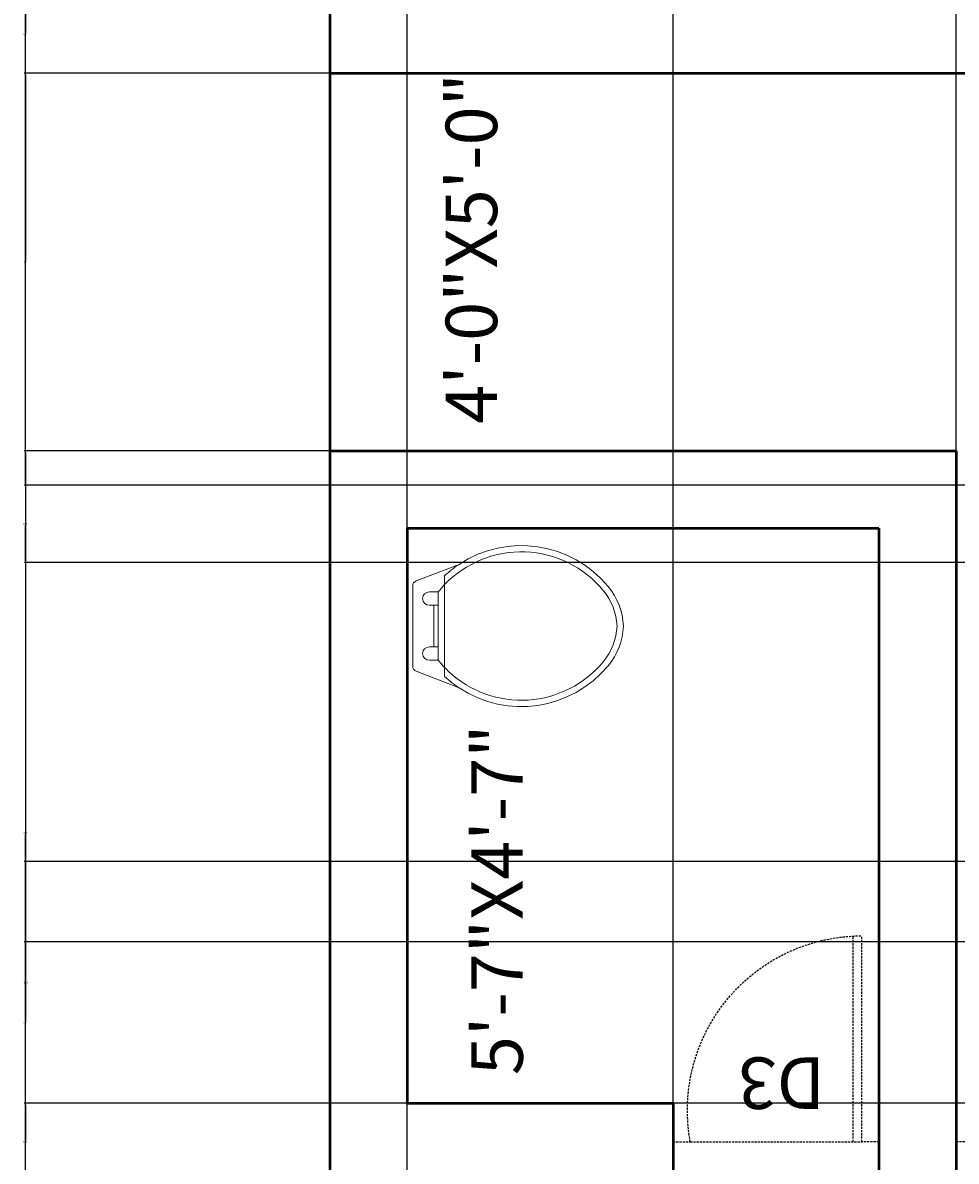
# Model space of a CAD drawing. Units: inches. Extents: x 3 to 576, y -689 to 51.
# Tile 14 of 21: x 3 to 111, y -261 to -128. Entities that reach past the tile are written whole.
import ezdxf

# ---------------------------------------------------------------- set-up
doc = ezdxf.new("R2010")
doc.units = ezdxf.units.IN
doc.header["$MEASUREMENT"] = 0
doc.linetypes.add('DASHED2', pattern=[0.375, 0.25, -0.125])
for name, color, linetype, lineweight in [('A-ANNO-DIMS', 2, 'Continuous', 18), ('A-ANNO-TEXT', 3, 'Continuous', 18), ('A-AREA-IDEN', 7, 'Continuous', 18), ('A-DOOR', 4, 'DASHED2', 25), ('A-FLOR-FIXT', 9, 'Continuous', 18), ('A-WALL', 7, 'Continuous', 50)]:
    doc.layers.add(name, color=color, linetype=linetype, lineweight=lineweight)
doc.styles.get("Standard").update_dxf_attribs({"font": 'arial.ttf'})
doc.dimstyles.get("Standard").update_dxf_attribs({"dimtxt": 0.18, "dimasz": 0.18, "dimexe": 0.18, "dimexo": 0.0625, "dimgap": 0.09, "dimtad": 0, "dimtih": 1, "dimtoh": 1, "dimdec": 0, "dimzin": 0, "dimdsep": 46, "dimlunit": 3, "dimtxsty": 'Standard', "dimcen": 0.09, "dimadec": 0, "dimazin": 0, "dimtfac": 1, "dimtdec": 0, "dimtofl": 0, "dimtmove": 0, "dimatfit": 3, "dimfxl": 1, "dimtolj": 1, "dimtzin": 0, "dimarcsym": 0})

# ---------------------------------------------------------------- blocks, each defined once
blk = doc.blocks.new('WC')
for p, q in [((3.72, 14.21), (3.72, 15.24)), ((3.72, 14.21), (3.72, 9.38)), ((3.72, 4.55), (3.72, 9.38)), ((3.72, 3.52), (3.72, 4.55))]:
    blk.add_line(p, q)
for points in [[(5.4, 16.57, -0.383919), (22.78, 13.99, -0.163732), (24.55, 9.38, -0.359733)], [(3.72, 14.21, -0.448546), (22.21, 13.53, -0.162618), (23.81, 9.38, -0.470877)], [(0, 9.38), (0, 14.07, -0.31031), (0.39, 14.64), (5.4, 16.57, -0.209071)], [(3.72, 15.24, -0.040937), (5.4, 16.57, -0.163732)], [(2.98, 13.36), (1.94, 13.36, 1), (1.94, 11.8), (2.48, 11.8)], [(2.98, 13.36, -0.022712), (3.72, 14.21, -0.162618)], [(2.98, 9.38), (2.98, 13.36, -0.476108)], [(0, 9.38), (0, 4.69, 0.31031), (0.39, 4.12), (5.4, 2.19, 0.209071)], [(2.98, 9.38), (2.98, 5.4, 0.022712)], [(4.22, 4.06, 0.431639), (22.21, 5.23, 0.162618), (23.81, 9.38, 0.470877)], [(5.4, 2.19, 0.383919), (22.78, 4.76, 0.163732), (24.55, 9.38, 0.359733)], [(2.98, 5.4), (1.94, 5.4, -1), (1.94, 6.96), (2.48, 6.96)], [(2.98, 5.4, 0.022712), (3.72, 4.55, 0.162618)], [(3.72, 4.55, 0.014165), (4.22, 4.06, 0.162618)], [(3.72, 3.52, 0.040937), (5.4, 2.19, 0.163732)]]:
    blk.add_lwpolyline(points, format="xyb")
for points in [[(2.48, 11.8), (2.48, 6.96)], [(2.48, 11.8), (2.98, 11.8)], [(2.48, 6.96), (2.98, 6.96)]]:
    blk.add_lwpolyline(points)
blk = doc.blocks.new('DOOR-SWING-750')
for p, q in [((24, 24), (24, 22)), ((24, 22), (24, 2)), ((24, 2), (0, 2)), ((24, 0), (24, 2))]:
    blk.add_line(p, q)
blk.add_arc((20.33, 2), 20.33, 79.6111, 180)
blk = doc.blocks.new('DOOR-900')
for p, q in [((34, 36), (0, 36)), ((2, 36), (2, 0)), ((36, 36), (34, 36))]:
    blk.add_line(p, q)
blk.add_arc((2, 32.22), 32.22, 270, 6.7329)
blk = doc.blocks.new('*D55')
at = {"layer": 'A-ANNO-DIMS', "color": 0, "lineweight": -2, "transparency": 16777216}
for p, q in [((47.23, -125.31), (2.66, -125.31)), ((2.84, -125.49), (2.84, -129.63)), ((2.84, -134.13), (2.84, -129.99)), ((38.23, -134.31), (2.66, -134.31))]:
    blk.add_line(p, q, dxfattribs=at)
at = {"layer": 'A-ANNO-DIMS', "color": 0, "transparency": 16777216}
for points in [[(2.81, -125.49), (2.87, -125.49), (2.84, -125.31)], [(2.81, -134.13), (2.87, -134.13), (2.84, -134.31)]]:
    blk.add_solid(points, dxfattribs=at)
at = {"layer": 'Defpoints', "color": 0, "transparency": 16777216}
for p in [(47.29, -125.31), (2.84, -134.31), (38.29, -134.31)]:
    blk.add_point(p, dxfattribs=at)
at = {"layer": 'A-ANNO-DIMS', "color": 0, "transparency": 16777216, "insert": (2.84, -129.81), "char_height": 0.18, "attachment_point": 5}
blk.add_mtext('\\A1;0\'-9"', dxfattribs=at)
blk = doc.blocks.new('*D56')
at = {"layer": 'A-ANNO-DIMS', "color": 0, "lineweight": -2, "transparency": 16777216}
for p, q in [((38.23, -134.31), (2.66, -134.31)), ((2.84, -134.49), (2.84, -156.13)), ((2.84, -178.13), (2.84, -156.49)), ((38.23, -178.31), (2.66, -178.31))]:
    blk.add_line(p, q, dxfattribs=at)
at = {"layer": 'A-ANNO-DIMS', "color": 0, "transparency": 16777216}
for points in [[(2.81, -134.49), (2.87, -134.49), (2.84, -134.31)], [(2.81, -178.13), (2.87, -178.13), (2.84, -178.31)]]:
    blk.add_solid(points, dxfattribs=at)
at = {"layer": 'Defpoints', "color": 0, "transparency": 16777216}
for p in [(38.29, -134.31), (2.84, -178.31), (38.29, -178.31)]:
    blk.add_point(p, dxfattribs=at)
at = {"layer": 'A-ANNO-DIMS', "color": 0, "transparency": 16777216, "insert": (2.84, -156.31), "char_height": 0.18, "attachment_point": 5}
blk.add_mtext('\\A1;3\'-8"', dxfattribs=at)
blk = doc.blocks.new('*D57')
at = {"layer": 'A-ANNO-DIMS', "color": 0, "lineweight": -2, "transparency": 16777216}
for p, q in [((38.23, -178.31), (2.66, -178.31)), ((2.84, -178.49), (2.84, -240.13)), ((2.84, -302.13), (2.84, -240.49)), ((47.23, -302.31), (2.66, -302.31))]:
    blk.add_line(p, q, dxfattribs=at)
at = {"layer": 'A-ANNO-DIMS', "color": 0, "transparency": 16777216}
for points in [[(2.81, -178.49), (2.87, -178.49), (2.84, -178.31)], [(2.81, -302.13), (2.87, -302.13), (2.84, -302.31)]]:
    blk.add_solid(points, dxfattribs=at)
at = {"layer": 'Defpoints', "color": 0, "transparency": 16777216}
for p in [(38.29, -178.31), (2.84, -302.31), (47.29, -302.31)]:
    blk.add_point(p, dxfattribs=at)
at = {"layer": 'A-ANNO-DIMS', "color": 0, "transparency": 16777216, "insert": (2.84, -240.31), "char_height": 0.18, "attachment_point": 5}
blk.add_mtext('\\A1;10\'-4"', dxfattribs=at)
blk = doc.blocks.new('*D65')
at = {"layer": 'A-ANNO-DIMS', "color": 0, "lineweight": -2, "transparency": 16777216}
for p, q in [((531.23, -50.31), (2.66, -50.31)), ((2.84, -50.49), (2.84, -116.13)), ((2.84, -182.13), (2.84, -116.49)), ((531.23, -182.31), (2.66, -182.31))]:
    blk.add_line(p, q, dxfattribs=at)
at = {"layer": 'A-ANNO-DIMS', "color": 0, "transparency": 16777216}
for points in [[(2.81, -50.49), (2.87, -50.49), (2.84, -50.31)], [(2.81, -182.13), (2.87, -182.13), (2.84, -182.31)]]:
    blk.add_solid(points, dxfattribs=at)
at = {"layer": 'Defpoints', "color": 0, "transparency": 16777216}
for p in [(531.29, -50.31), (2.84, -182.31), (531.29, -182.31)]:
    blk.add_point(p, dxfattribs=at)
at = {"layer": 'A-ANNO-DIMS', "color": 0, "transparency": 16777216, "insert": (2.84, -116.31), "char_height": 0.18, "attachment_point": 5}
blk.add_mtext('\\A1;11\'-0"', dxfattribs=at)
blk = doc.blocks.new('*D66')
at = {"layer": 'A-ANNO-DIMS', "color": 0, "lineweight": -2, "transparency": 16777216}
for p, q in [((531.23, -182.31), (2.66, -182.31)), ((2.84, -182.49), (2.84, -186.63)), ((2.84, -191.13), (2.84, -186.99)), ((531.23, -191.31), (2.66, -191.31))]:
    blk.add_line(p, q, dxfattribs=at)
at = {"layer": 'A-ANNO-DIMS', "color": 0, "transparency": 16777216}
for points in [[(2.81, -182.49), (2.87, -182.49), (2.84, -182.31)], [(2.81, -191.13), (2.87, -191.13), (2.84, -191.31)]]:
    blk.add_solid(points, dxfattribs=at)
at = {"layer": 'Defpoints', "color": 0, "transparency": 16777216}
for p in [(531.29, -182.31), (2.84, -191.31), (531.29, -191.31)]:
    blk.add_point(p, dxfattribs=at)
at = {"layer": 'A-ANNO-DIMS', "color": 0, "transparency": 16777216, "insert": (2.84, -186.81), "char_height": 0.18, "attachment_point": 5}
blk.add_mtext('\\A1;0\'-9"', dxfattribs=at)
blk = doc.blocks.new('*D67')
at = {"layer": 'A-ANNO-DIMS', "color": 0, "lineweight": -2, "transparency": 16777216}
for p, q in [((531.23, -191.31), (2.66, -191.31)), ((2.84, -191.49), (2.84, -222.63)), ((2.84, -254.13), (2.84, -222.99)), ((531.23, -254.31), (2.66, -254.31))]:
    blk.add_line(p, q, dxfattribs=at)
at = {"layer": 'A-ANNO-DIMS', "color": 0, "transparency": 16777216}
for points in [[(2.81, -191.49), (2.87, -191.49), (2.84, -191.31)], [(2.81, -254.13), (2.87, -254.13), (2.84, -254.31)]]:
    blk.add_solid(points, dxfattribs=at)
at = {"layer": 'Defpoints', "color": 0, "transparency": 16777216}
for p in [(531.29, -191.31), (2.84, -254.31), (531.29, -254.31)]:
    blk.add_point(p, dxfattribs=at)
at = {"layer": 'A-ANNO-DIMS', "color": 0, "transparency": 16777216, "insert": (2.84, -222.81), "char_height": 0.18, "attachment_point": 5}
blk.add_mtext('\\A1;5\'-3"', dxfattribs=at)
blk = doc.blocks.new('*D68')
at = {"layer": 'A-ANNO-DIMS', "color": 0, "lineweight": -2, "transparency": 16777216}
for p, q in [((531.23, -254.31), (2.66, -254.31)), ((2.84, -254.49), (2.84, -258.63)), ((2.84, -263.13), (2.84, -258.99)), ((531.23, -263.31), (2.66, -263.31))]:
    blk.add_line(p, q, dxfattribs=at)
at = {"layer": 'A-ANNO-DIMS', "color": 0, "transparency": 16777216}
for points in [[(2.81, -254.49), (2.87, -254.49), (2.84, -254.31)], [(2.81, -263.13), (2.87, -263.13), (2.84, -263.31)]]:
    blk.add_solid(points, dxfattribs=at)
at = {"layer": 'Defpoints', "color": 0, "transparency": 16777216}
for p in [(531.29, -254.31), (2.84, -263.31), (531.29, -263.31)]:
    blk.add_point(p, dxfattribs=at)
at = {"layer": 'A-ANNO-DIMS', "color": 0, "transparency": 16777216, "insert": (2.84, -258.81), "char_height": 0.18, "attachment_point": 5}
blk.add_mtext('\\A1;0\'-9"', dxfattribs=at)
blk = doc.blocks.new('*D89')
at = {"layer": 'A-ANNO-DIMS', "color": 0, "lineweight": -2, "transparency": 16777216}
for p, q in [((170.74, -226.15), (2.66, -226.15)), ((2.84, -226.33), (2.84, -240.05)), ((2.84, -254.13), (2.84, -240.41)), ((170.74, -254.31), (2.66, -254.31))]:
    blk.add_line(p, q, dxfattribs=at)
at = {"layer": 'A-ANNO-DIMS', "color": 0, "transparency": 16777216}
for points in [[(2.81, -226.33), (2.87, -226.33), (2.84, -226.15)], [(2.81, -254.13), (2.87, -254.13), (2.84, -254.31)]]:
    blk.add_solid(points, dxfattribs=at)
at = {"layer": 'Defpoints', "color": 0, "transparency": 16777216}
for p in [(2.84, -226.15), (170.8, -226.15), (170.8, -254.31)]:
    blk.add_point(p, dxfattribs=at)
at = {"layer": 'A-ANNO-DIMS', "color": 0, "transparency": 16777216, "insert": (2.84, -240.23), "char_height": 0.18, "attachment_point": 5}
blk.add_mtext('\\A1;2\'-4"', dxfattribs=at)
blk = doc.blocks.new('*D101')
at = {"layer": 'A-ANNO-DIMS', "color": 0, "lineweight": -2, "transparency": 16777216}
for p, q in [((47.29, -254.25), (47.29, 51.32)), ((47.47, 51.14), (62.46, 51.14)), ((78.11, 51.14), (63.12, 51.14)), ((78.29, -254.25), (78.29, 51.32))]:
    blk.add_line(p, q, dxfattribs=at)
at = {"layer": 'A-ANNO-DIMS', "color": 0, "transparency": 16777216}
for points in [[(47.47, 51.17), (47.47, 51.11), (47.29, 51.14)], [(78.11, 51.17), (78.11, 51.11), (78.29, 51.14)]]:
    blk.add_solid(points, dxfattribs=at)
at = {"layer": 'Defpoints', "color": 0, "transparency": 16777216}
for p in [(78.29, 51.14), (47.29, -254.31), (78.29, -254.31)]:
    blk.add_point(p, dxfattribs=at)
at = {"layer": 'A-ANNO-DIMS', "color": 0, "transparency": 16777216, "insert": (62.79, 51.14), "char_height": 0.18, "attachment_point": 5}
blk.add_mtext('\\A1;2\'-7"', dxfattribs=at)
blk = doc.blocks.new('*D119')
at = {"layer": 'A-ANNO-DIMS', "color": 0, "lineweight": -2, "transparency": 16777216}
for p, q in [((47.29, -311.25), (47.29, 51.32)), ((47.47, 51.14), (78.96, 51.14)), ((111.11, 51.14), (79.62, 51.14)), ((111.29, -311.25), (111.29, 51.32))]:
    blk.add_line(p, q, dxfattribs=at)
at = {"layer": 'A-ANNO-DIMS', "color": 0, "transparency": 16777216}
for points in [[(47.47, 51.17), (47.47, 51.11), (47.29, 51.14)], [(111.11, 51.17), (111.11, 51.11), (111.29, 51.14)]]:
    blk.add_solid(points, dxfattribs=at)
at = {"layer": 'Defpoints', "color": 0, "transparency": 16777216}
for p in [(111.29, 51.14), (47.29, -311.31), (111.29, -311.31)]:
    blk.add_point(p, dxfattribs=at)
at = {"layer": 'A-ANNO-DIMS', "color": 0, "transparency": 16777216, "insert": (79.29, 51.14), "char_height": 0.18, "attachment_point": 5}
blk.add_mtext('\\A1;5\'-4"', dxfattribs=at)
blk = doc.blocks.new('*D123')
at = {"layer": 'A-ANNO-DIMS', "color": 0, "lineweight": -2, "transparency": 16777216}
for p, q in [((513.55, -235.5), (2.66, -235.5)), ((2.84, -235.68), (2.84, -244.72)), ((2.84, -254.13), (2.84, -245.08)), ((531.23, -254.31), (2.66, -254.31))]:
    blk.add_line(p, q, dxfattribs=at)
at = {"layer": 'A-ANNO-DIMS', "color": 0, "transparency": 16777216}
for points in [[(2.81, -235.68), (2.87, -235.68), (2.84, -235.5)], [(2.81, -254.13), (2.87, -254.13), (2.84, -254.31)]]:
    blk.add_solid(points, dxfattribs=at)
at = {"layer": 'Defpoints', "color": 0, "transparency": 16777216}
for p in [(513.61, -235.5), (2.84, -254.31), (531.29, -254.31)]:
    blk.add_point(p, dxfattribs=at)
at = {"layer": 'A-ANNO-DIMS', "color": 0, "transparency": 16777216, "insert": (2.84, -244.9), "char_height": 0.18, "attachment_point": 5}
blk.add_mtext('\\A1;1\'-7"', dxfattribs=at)

msp = doc.modelspace()

# ---------------------------------------------------------------- linework, layer by layer
at = {"layer": 'A-DOOR'}
msp.add_line((99.29, -258.81), (99.29, -234.81), dxfattribs=at)
at = {"layer": 'A-WALL'}
for p, q in [((38.29, 15.69), (38.29, -653.31)), ((38.29, -134.31), (255.29, -134.31)), ((38.29, -178.31), (102.29, -178.31)), ((102.29, -178.31), (111.29, -178.31)), ((111.29, -178.31), (111.29, -263.31)), ((47.29, -187.31), (47.29, -254.31)), ((47.29, -187.31), (102.29, -187.31)), ((102.29, -187.31), (102.29, -263.31)), ((47.29, -254.31), (78.29, -254.31)), ((47.29, -254.31), (78.29, -254.31)), ((78.29, -254.31), (78.29, -263.31))]:
    msp.add_line(p, q, dxfattribs=at)

# ---------------------------------------------------------------- block references
at = {"layer": 'A-DOOR', "extrusion": (0, 0, -1), "zscale": -1}
for name, p, rotation in [('DOOR-900', (-111.29, -222.81), 180), ('DOOR-SWING-750', (-102.29, -234.81), 269.9999999999999)]:
    msp.add_blockref(name, p, dxfattribs=dict(at, rotation=rotation))
at = {"layer": 'A-FLOR-FIXT'}
msp.add_blockref('WC', (47.95, -208.1), dxfattribs=at)

# ---------------------------------------------------------------- texts
at = {"layer": 'A-ANNO-TEXT', "insert": (96.01, -254.98), "char_height": 6, "attachment_point": 1, "rotation": 180}
msp.add_mtext_dynamic_manual_height_columns('D3', width=0.7543, gutter_width=1, heights=[0], dxfattribs=at)
at = {"layer": 'A-AREA-IDEN', "char_height": 6, "attachment_point": 1, "rotation": 90}
for s, insert in [('4\'-0"X5\'-0"', (51.79, -175.15)), ('5\'-7"X4\'-7"', (54.78, -251.04))]:
    msp.add_mtext(s, dxfattribs=dict(at, insert=insert))

# ---------------------------------------------------------------- dimensions: what is measured, and where the dimension line sits
at = {"layer": 'A-ANNO-DIMS'}
for base, p1, p2, picture, middle in [((78.29, 51.14), (47.29, -254.31), (78.29, -254.31), '*D101', (62.79, 51.14)), ((111.29, 51.14), (47.29, -311.31), (111.29, -311.31), '*D119', (79.29, 51.14))]:
    dim = msp.add_linear_dim(base=base, p1=p1, p2=p2, dimstyle='Standard', override={"dimdec": 1, "dimlfac": 1, "dimrnd": 0, "dimzin": 1, "dimdsep": 46, "dimlunit": 4, "dimfrac": 2}, dxfattribs=at)
    dim.commit()
    dim.dimension.update_dxf_attribs({"geometry": picture, "text_midpoint": middle})
for base, p1, p2, picture, middle in [((2.84, -182.31), (531.29, -50.31), (531.29, -182.31), '*D65', (2.84, -116.31)), ((2.84, -134.31), (47.29, -125.31), (38.29, -134.31), '*D55', (2.84, -129.81)), ((2.84, -178.31), (38.29, -134.31), (38.29, -178.31), '*D56', (2.84, -156.31)), ((2.84, -302.31), (38.29, -178.31), (47.29, -302.31), '*D57', (2.84, -240.31)), ((2.84, -191.31), (531.29, -182.31), (531.29, -191.31), '*D66', (2.84, -186.81)), ((2.84, -254.31), (531.29, -191.31), (531.29, -254.31), '*D67', (2.84, -222.81)), ((2.84, -226.15), (170.8, -254.31), (170.8, -226.15), '*D89', (2.84, -240.23)), ((2.84, -254.31), (513.61, -235.5), (531.29, -254.31), '*D123', (2.84, -244.9)), ((2.84, -263.31), (531.29, -254.31), (531.29, -263.31), '*D68', (2.84, -258.81))]:
    dim = msp.add_linear_dim(base=base, p1=p1, p2=p2, angle=90, dimstyle='Standard', override={"dimdec": 1, "dimlfac": 1, "dimrnd": 0, "dimzin": 1, "dimdsep": 46, "dimlunit": 4, "dimfrac": 2}, dxfattribs=at)
    dim.commit()
    dim.dimension.update_dxf_attribs({"geometry": picture, "text_midpoint": middle})

doc.saveas('drawing.dxf')
